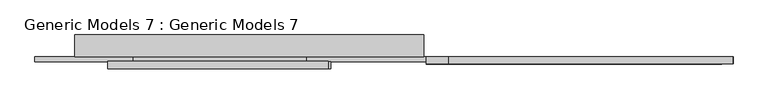
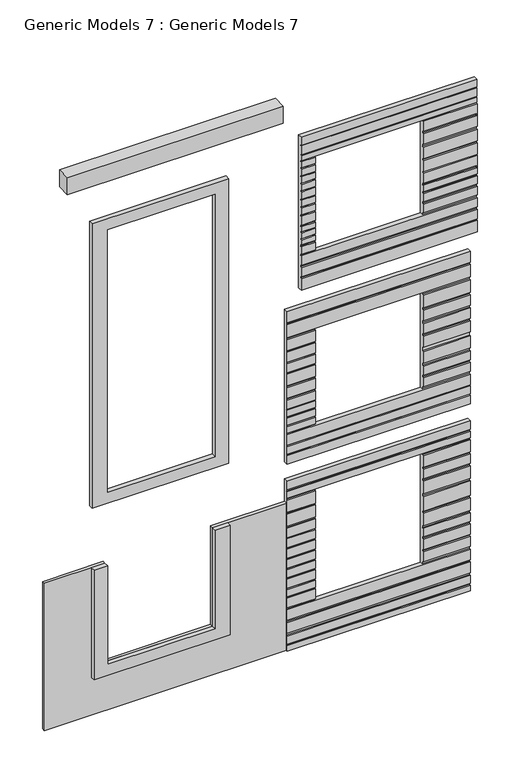
"""IFC4 building model written with IfcOpenShell, lengths in millimetres: proxy geometry, Generic Models 7 : Generic Models 7."""

from ifc_helpers import new_model, si_unit, frame, origin, place, context, project, spatial, polyline, outline, extrude, faceted_brep, source, transform, mapped, element, save


def generic_models_7_generic_models_7_680a3b92(model_context):
    return source(origin(), model_context, "Body", "SolidModel", [
        extrude(outline(polyline([(-16196.191855, -13854.1538163), (-19866.491855, -13854.1538163), (-19866.491855, -13625.5538163), (-16196.191855, -13625.5538163), (-16196.191855, -13854.1538163)])), frame((0.0, 0.0, 9448.8), z_axis=(0.0, 0.0, 1.0), x_axis=(1.0, 0.0, 0.0)), (0.0, 0.0, 1.0), 304.8),
        extrude(outline(polyline([(2645.3232141, -19485.491855), (675.8427781, -19485.491855), (675.8427781, -17174.091855), (2645.3232141, -17174.091855), (2645.3232141, -17428.091855), (874.5903603, -17428.091855), (874.5903603, -19256.891855), (2645.3232141, -19256.891855), (2645.3232141, -19485.491855)])), frame((0.0, -13981.1538163, 0.0), z_axis=(0.0, 1.0, 0.0), x_axis=(0.0, 0.0, 1.0)), (0.0, 0.0, 1.0), 76.2),
        faceted_brep([(-13059.291855, -13930.3538163, 3047.830136), (-16170.791855, -13930.3538163, 3047.830136), (-16170.791855, -13930.3538163, 2895.4466758), (-13059.291855, -13930.3538163, 2895.4466758), (-16170.791855, -13930.3538163, 0.0), (-13059.291855, -13930.3538163, 0.0), (-13059.291855, -13930.3538163, 95.1342014), (-16170.791855, -13930.3538163, 95.1342014), (-13859.391855, -13930.3538163, 2703.7494971), (-13859.391855, -13930.3538163, 2491.4485326), (-13059.291855, -13930.3538163, 2491.4485326), (-13059.291855, -13930.3538163, 2703.7494971), (-13859.391855, -13930.3538163, 2458.2818029), (-13859.391855, -13930.3538163, 2283.5976577), (-13059.291855, -13930.3538163, 2283.5976577), (-13059.291855, -13930.3538163, 2458.2818029), (-13859.391855, -13930.3538163, 2241.6081652), (-13859.391855, -13930.3538163, 2015.4004334), (-13059.291855, -13930.3538163, 2015.4004334), (-13059.291855, -13930.3538163, 2241.6081652), (-13859.391855, -13930.3538163, 1968.3766728), (-13859.391855, -13930.3538163, 1706.6714658), (-13059.291855, -13930.3538163, 1706.6714658), (-13059.291855, -13930.3538163, 1968.3766728), (-13859.391855, -13930.3538163, 1667.5135795), (-13859.391855, -13930.3538163, 1443.0083646), (-13059.291855, -13930.3538163, 1443.0083646), (-13059.291855, -13930.3538163, 1667.5135795), (-13859.391855, -13930.3538163, 1396.018901), (-13859.391855, -13930.3538163, 1241.8672624), (-13059.291855, -13930.3538163, 1241.8672624), (-13059.291855, -13930.3538163, 1396.018901), (-13859.391855, -13930.3538163, 978.3347801), (-13859.391855, -13930.3538163, 792.9874515), (-13059.291855, -13930.3538163, 792.9874515), (-13059.291855, -13930.3538163, 978.3347801), (-13859.391855, -13930.3538163, 1200.2294693), (-13859.391855, -13930.3538163, 1009.6610892), (-13059.291855, -13930.3538163, 1009.6610892), (-13059.291855, -13930.3538163, 1200.2294693), (-15688.191855, -13930.3538163, 2491.4485326), (-15688.191855, -13930.3538163, 2714.9644319), (-16170.791855, -13930.3538163, 2714.9644319), (-16170.791855, -13930.3538163, 2491.4485326), (-15688.191855, -13930.3538163, 2241.6081652), (-15688.191855, -13930.3538163, 2458.2818029), (-16170.791855, -13930.3538163, 2458.2818029), (-16170.791855, -13930.3538163, 2241.6081652), (-15688.191855, -13930.3538163, 2040.597682), (-15688.191855, -13930.3538163, 2205.0608046), (-16170.791855, -13930.3538163, 2205.0608046), (-16170.791855, -13930.3538163, 2040.597682), (-15688.191855, -13930.3538163, 1854.7223265), (-15688.191855, -13930.3538163, 2015.4004334), (-16170.791855, -13930.3538163, 2015.4004334), (-16170.791855, -13930.3538163, 1854.7223265), (-15688.191855, -13930.3538163, 1670.8505124), (-15688.191855, -13930.3538163, 1829.7520801), (-16170.791855, -13930.3538163, 1829.7520801), (-16170.791855, -13930.3538163, 1670.8505124), (-15688.191855, -13930.3538163, 1491.5187431), (-15688.191855, -13930.3538163, 1641.3402213), (-16170.791855, -13930.3538163, 1641.3402213), (-16170.791855, -13930.3538163, 1491.5187431), (-15688.191855, -13930.3538163, 1322.6616071), (-15688.191855, -13930.3538163, 1464.2784744), (-16170.791855, -13930.3538163, 1464.2784744), (-16170.791855, -13930.3538163, 1322.6616071), (-15688.191855, -13930.3538163, 1130.5851822), (-15688.191855, -13930.3538163, 1291.7567723), (-16170.791855, -13930.3538163, 1291.7567723), (-16170.791855, -13930.3538163, 1130.5851822), (-15688.191855, -13930.3538163, 776.4616885), (-15688.191855, -13930.3538163, 951.253413), (-16170.791855, -13930.3538163, 951.253413), (-16170.791855, -13930.3538163, 776.4616885), (-15688.191855, -13930.3538163, 978.4936817), (-15688.191855, -13930.3538163, 1105.6149359), (-16170.791855, -13930.3538163, 1105.6149359), (-16170.791855, -13930.3538163, 978.4936817), (-16170.791855, -13930.3538163, 512.7768801), (-16170.791855, -13930.3538163, 322.2032789), (-13059.291855, -13930.3538163, 322.2032789), (-13059.291855, -13930.3538163, 512.7768801), (-16170.791855, -13930.3538163, 270.5895953), (-16170.791855, -13930.3538163, 127.6593944), (-13059.291855, -13930.3538163, 127.6593944), (-13059.291855, -13930.3538163, 270.5895953), (-16170.791855, -13930.3538163, 2743.3706019), (-13059.291855, -13930.3538163, 2743.3706019), (-13059.291855, -13930.3538163, 2861.3685959), (-16170.791855, -13930.3538163, 2861.3685959), (-13059.291855, -13930.3538163, 741.3661492), (-16170.791855, -13930.3538163, 741.3661492), (-16170.791855, -13930.3538163, 556.4499971), (-13059.291855, -13930.3538163, 556.4499971), (-16170.791855, -13854.1538163, 3047.830136), (-13059.291855, -13854.1538163, 3047.830136), (-13059.291855, -13854.1538163, 0.0), (-16170.791855, -13854.1538163, 0.0), (-15688.191855, -13854.1538163, 2743.3706019), (-15688.191855, -13854.1538163, 741.3661492), (-13859.391855, -13854.1538163, 741.3661492), (-13859.391855, -13854.1538163, 2743.3706019), (-16170.791855, -13904.9538163, 95.1342014), (-16170.791855, -13904.9538163, 127.6593944), (-16170.791855, -13904.9538163, 270.5895953), (-16170.791855, -13904.9538163, 322.2032789), (-16170.791855, -13904.9538163, 512.7768801), (-16170.791855, -13904.9538163, 556.4499971), (-16170.791855, -13904.9538163, 741.3661492), (-16170.791855, -13904.9538163, 776.4616885), (-16170.791855, -13904.9538163, 951.253413), (-16170.791855, -13904.9538163, 978.4936817), (-16170.791855, -13904.9538163, 1105.6149359), (-16170.791855, -13904.9538163, 1130.5851822), (-16170.791855, -13904.9538163, 1291.7567723), (-16170.791855, -13904.9538163, 1322.6616071), (-16170.791855, -13904.9538163, 1464.2784744), (-16170.791855, -13904.9538163, 1491.5187431), (-16170.791855, -13904.9538163, 1641.3402213), (-16170.791855, -13904.9538163, 1670.8505124), (-16170.791855, -13904.9538163, 1829.7520801), (-16170.791855, -13904.9538163, 1854.7223265), (-16170.791855, -13904.9538163, 2015.4004334), (-16170.791855, -13904.9538163, 2040.597682), (-16170.791855, -13904.9538163, 2205.0608046), (-16170.791855, -13904.9538163, 2241.6081652), (-16170.791855, -13904.9538163, 2458.2818029), (-16170.791855, -13904.9538163, 2491.4485326), (-16170.791855, -13904.9538163, 2714.9644319), (-16170.791855, -13904.9538163, 2743.3706019), (-16170.791855, -13904.9538163, 2861.3685959), (-16170.791855, -13904.9538163, 2895.4466758), (-15688.191855, -13904.9538163, 2743.3706019), (-15688.191855, -13904.9538163, 2714.9644319), (-15688.191855, -13904.9538163, 2491.4485326), (-15688.191855, -13904.9538163, 2458.2818029), (-15688.191855, -13904.9538163, 2241.6081652), (-15688.191855, -13904.9538163, 2205.0608046), (-15688.191855, -13904.9538163, 2040.597682), (-15688.191855, -13904.9538163, 2015.4004334), (-15688.191855, -13904.9538163, 1854.7223265), (-15688.191855, -13904.9538163, 1829.7520801), (-15688.191855, -13904.9538163, 1670.8505124), (-15688.191855, -13904.9538163, 1641.3402213), (-15688.191855, -13904.9538163, 1491.5187431), (-15688.191855, -13904.9538163, 1464.2784744), (-15688.191855, -13904.9538163, 1322.6616071), (-15688.191855, -13904.9538163, 1291.7567723), (-15688.191855, -13904.9538163, 1130.5851822), (-15688.191855, -13904.9538163, 1105.6149359), (-15688.191855, -13904.9538163, 978.4936817), (-15688.191855, -13904.9538163, 951.253413), (-15688.191855, -13904.9538163, 776.4616885), (-15688.191855, -13904.9538163, 741.3661492), (-13859.391855, -13904.9538163, 2743.3706019), (-13059.291855, -13904.9538163, 2743.3706019), (-13059.291855, -13904.9538163, 2895.4466758), (-13059.291855, -13904.9538163, 2861.3685959), (-13059.291855, -13904.9538163, 2703.7494971), (-13059.291855, -13904.9538163, 2491.4485326), (-13059.291855, -13904.9538163, 2458.2818029), (-13059.291855, -13904.9538163, 2283.5976577), (-13059.291855, -13904.9538163, 2241.6081652), (-13059.291855, -13904.9538163, 2015.4004334), (-13059.291855, -13904.9538163, 1968.3766728), (-13059.291855, -13904.9538163, 1706.6714658), (-13059.291855, -13904.9538163, 1667.5135795), (-13059.291855, -13904.9538163, 1443.0083646), (-13059.291855, -13904.9538163, 1396.018901), (-13059.291855, -13904.9538163, 1241.8672624), (-13059.291855, -13904.9538163, 1200.2294693), (-13059.291855, -13904.9538163, 1009.6610892), (-13059.291855, -13904.9538163, 978.3347801), (-13059.291855, -13904.9538163, 792.9874515), (-13059.291855, -13904.9538163, 741.3661492), (-13059.291855, -13904.9538163, 556.4499971), (-13059.291855, -13904.9538163, 512.7768801), (-13059.291855, -13904.9538163, 322.2032789), (-13059.291855, -13904.9538163, 270.5895953), (-13059.291855, -13904.9538163, 127.6593944), (-13059.291855, -13904.9538163, 95.1342014), (-13859.391855, -13904.9538163, 741.3661492), (-13859.391855, -13904.9538163, 792.9874515), (-13859.391855, -13904.9538163, 978.3347801), (-13859.391855, -13904.9538163, 1009.6610892), (-13859.391855, -13904.9538163, 1200.2294693), (-13859.391855, -13904.9538163, 1241.8672624), (-13859.391855, -13904.9538163, 1396.018901), (-13859.391855, -13904.9538163, 1443.0083646), (-13859.391855, -13904.9538163, 1667.5135795), (-13859.391855, -13904.9538163, 1706.6714658), (-13859.391855, -13904.9538163, 1968.3766728), (-13859.391855, -13904.9538163, 2015.4004334), (-13859.391855, -13904.9538163, 2241.6081652), (-13859.391855, -13904.9538163, 2283.5976577), (-13859.391855, -13904.9538163, 2458.2818029), (-13859.391855, -13904.9538163, 2491.4485326), (-13859.391855, -13904.9538163, 2703.7494971)], [[[0, 1, 2, 3]], [[4, 5, 6, 7]], [[8, 9, 10, 11]], [[12, 13, 14, 15]], [[16, 17, 18, 19]], [[20, 21, 22, 23]], [[24, 25, 26, 27]], [[28, 29, 30, 31]], [[32, 33, 34, 35]], [[36, 37, 38, 39]], [[40, 41, 42, 43]], [[44, 45, 46, 47]], [[48, 49, 50, 51]], [[52, 53, 54, 55]], [[56, 57, 58, 59]], [[60, 61, 62, 63]], [[64, 65, 66, 67]], [[68, 69, 70, 71]], [[72, 73, 74, 75]], [[76, 77, 78, 79]], [[80, 81, 82, 83]], [[84, 85, 86, 87]], [[88, 89, 90, 91]], [[92, 93, 94, 95]], [[96, 97, 98, 99], [100, 101, 102, 103]], [[99, 4, 7, 104, 105, 85, 84, 106, 107, 81, 80, 108, 109, 94, 93, 110, 111, 75, 74, 112, 113, 79, 78, 114, 115, 71, 70, 116, 117, 67, 66, 118, 119, 63, 62, 120, 121, 59, 58, 122, 123, 55, 54, 124, 125, 51, 50, 126, 127, 47, 46, 128, 129, 43, 42, 130, 131, 88, 91, 132, 133, 2, 1, 96]], [[4, 99, 98, 5]], [[101, 100, 134, 135, 41, 40, 136, 137, 45, 44, 138, 139, 49, 48, 140, 141, 53, 52, 142, 143, 57, 56, 144, 145, 61, 60, 146, 147, 65, 64, 148, 149, 69, 68, 150, 151, 77, 76, 152, 153, 73, 72, 154, 155]], [[1, 0, 97, 96]], [[88, 131, 134, 100, 103, 156, 157, 89]], [[97, 0, 3, 158, 159, 90, 89, 157, 160, 11, 10, 161, 162, 15, 14, 163, 164, 19, 18, 165, 166, 23, 22, 167, 168, 27, 26, 169, 170, 31, 30, 171, 172, 39, 38, 173, 174, 35, 34, 175, 176, 92, 95, 177, 178, 83, 82, 179, 180, 87, 86, 181, 182, 6, 5, 98]], [[92, 176, 183, 102, 101, 155, 110, 93]], [[103, 102, 183, 184, 33, 32, 185, 186, 37, 36, 187, 188, 29, 28, 189, 190, 25, 24, 191, 192, 21, 20, 193, 194, 17, 16, 195, 196, 13, 12, 197, 198, 9, 8, 199, 156]], [[157, 156, 199, 160]], [[110, 155, 154, 111]], [[158, 133, 132, 159]], [[130, 135, 134, 131]], [[136, 129, 128, 137]], [[138, 127, 126, 139]], [[140, 125, 124, 141]], [[142, 123, 122, 143]], [[144, 121, 120, 145]], [[146, 119, 118, 147]], [[148, 117, 116, 149]], [[150, 115, 114, 151]], [[152, 113, 112, 153]], [[161, 198, 197, 162]], [[163, 196, 195, 164]], [[165, 194, 193, 166]], [[167, 192, 191, 168]], [[175, 184, 183, 176]], [[169, 190, 189, 170]], [[171, 188, 187, 172]], [[173, 186, 185, 174]], [[177, 109, 108, 178]], [[179, 107, 106, 180]], [[181, 105, 104, 182]], [[159, 132, 91, 90]], [[133, 158, 3, 2]], [[135, 130, 42, 41]], [[160, 199, 8, 11]], [[137, 128, 46, 45]], [[129, 136, 40, 43]], [[139, 126, 50, 49]], [[127, 138, 44, 47]], [[141, 124, 54, 53]], [[125, 140, 48, 51]], [[143, 122, 58, 57]], [[123, 142, 52, 55]], [[145, 120, 62, 61]], [[121, 144, 56, 59]], [[147, 118, 66, 65]], [[119, 146, 60, 63]], [[111, 154, 72, 75]], [[149, 116, 70, 69]], [[117, 148, 64, 67]], [[151, 114, 78, 77]], [[115, 150, 68, 71]], [[153, 112, 74, 73]], [[113, 152, 76, 79]], [[162, 197, 12, 15]], [[198, 161, 10, 9]], [[164, 195, 16, 19]], [[196, 163, 14, 13]], [[166, 193, 20, 23]], [[194, 165, 18, 17]], [[168, 191, 24, 27]], [[192, 167, 22, 21]], [[184, 175, 34, 33]], [[170, 189, 28, 31]], [[190, 169, 26, 25]], [[172, 187, 36, 39]], [[188, 171, 30, 29]], [[174, 185, 32, 35]], [[186, 173, 38, 37]], [[178, 108, 80, 83]], [[109, 177, 95, 94]], [[180, 106, 84, 87]], [[107, 179, 82, 81]], [[182, 104, 7, 6]], [[105, 181, 86, 85]]]),
        faceted_brep([(-13059.291855, -13930.3538163, 6096.0), (-16170.791855, -13930.3538163, 6096.0), (-16170.791855, -13930.3538163, 5900.4772221), (-13059.291855, -13930.3538163, 5900.4772221), (-16170.791855, -13930.3538163, 3352.8), (-13059.291855, -13930.3538163, 3352.8), (-13059.291855, -13930.3538163, 3510.1812657), (-16170.791855, -13930.3538163, 3510.1812657), (-13859.391855, -13930.3538163, 5586.1430956), (-13859.391855, -13930.3538163, 5358.1855285), (-13059.291855, -13930.3538163, 5358.1855285), (-13059.291855, -13930.3538163, 5586.1430956), (-13859.391855, -13930.3538163, 5316.1560639), (-13859.391855, -13930.3538163, 5121.0192637), (-13059.291855, -13930.3538163, 5121.0192637), (-13059.291855, -13930.3538163, 5316.1560639), (-13859.391855, -13930.3538163, 5075.9876944), (-13859.391855, -13930.3538163, 4892.8593127), (-13059.291855, -13930.3538163, 4892.8593127), (-13059.291855, -13930.3538163, 5075.9876944), (-13859.391855, -13930.3538163, 4847.8277434), (-13859.391855, -13930.3538163, 4647.2829369), (-13059.291855, -13930.3538163, 4647.2829369), (-13059.291855, -13930.3538163, 4847.8277434), (-13859.391855, -13930.3538163, 4572.0), (-13859.391855, -13930.3538163, 4358.4846906), (-13059.291855, -13930.3538163, 4358.4846906), (-13059.291855, -13930.3538163, 4572.0), (-13859.391855, -13930.3538163, 4103.305798), (-13859.391855, -13930.3538163, 3938.190044), (-13059.291855, -13930.3538163, 3938.190044), (-13059.291855, -13930.3538163, 4103.305798), (-13859.391855, -13930.3538163, 4307.4489121), (-13859.391855, -13930.3538163, 4145.3352627), (-13059.291855, -13930.3538163, 4145.3352627), (-13059.291855, -13930.3538163, 4307.4489121), (-15688.191855, -13930.3538163, 5394.7918514), (-15688.191855, -13930.3538163, 5596.5851986), (-16170.791855, -13930.3538163, 5596.5851986), (-16170.791855, -13930.3538163, 5394.7918514), (-15688.191855, -13930.3538163, 5189.2435919), (-15688.191855, -13930.3538163, 5368.6865939), (-16170.791855, -13930.3538163, 5368.6865939), (-16170.791855, -13930.3538163, 5189.2435919), (-15688.191855, -13930.3538163, 5003.2129882), (-15688.191855, -13930.3538163, 5165.065585), (-16170.791855, -13930.3538163, 5165.065585), (-16170.791855, -13930.3538163, 5003.2129882), (-15688.191855, -13930.3538163, 4768.0829809), (-15688.191855, -13930.3538163, 4971.8866791), (-16170.791855, -13930.3538163, 4971.8866791), (-16170.791855, -13930.3538163, 4768.0829809), (-15688.191855, -13930.3538163, 4543.4835442), (-15688.191855, -13930.3538163, 4734.1666909), (-16170.791855, -13930.3538163, 4734.1666909), (-16170.791855, -13930.3538163, 4543.4835442), (-15688.191855, -13930.3538163, 4346.2982993), (-15688.191855, -13930.3538163, 4510.8707461), (-16170.791855, -13930.3538163, 4510.8707461), (-16170.791855, -13930.3538163, 4346.2982993), (-15688.191855, -13930.3538163, 4212.2061738), (-15688.191855, -13930.3538163, 4324.3827349), (-16170.791855, -13930.3538163, 4324.3827349), (-16170.791855, -13930.3538163, 4212.2061738), (-15688.191855, -13930.3538163, 3915.2580645), (-15688.191855, -13930.3538163, 4034.0671597), (-16170.791855, -13930.3538163, 4034.0671597), (-16170.791855, -13930.3538163, 3915.2580645), (-15688.191855, -13930.3538163, 4059.1404662), (-15688.191855, -13930.3538163, 4183.0263018), (-16170.791855, -13930.3538163, 4183.0263018), (-16170.791855, -13930.3538163, 4059.1404662), (-16170.791855, -13930.3538163, 3674.3162613), (-16170.791855, -13930.3538163, 3536.2157608), (-13059.291855, -13930.3538163, 3536.2157608), (-13059.291855, -13930.3538163, 3674.3162613), (-16170.791855, -13930.3538163, 5631.310527), (-13059.291855, -13930.3538163, 5631.310527), (-13059.291855, -13930.3538163, 5862.3466577), (-16170.791855, -13930.3538163, 5862.3466577), (-13059.291855, -13930.3538163, 3888.7401376), (-16170.791855, -13930.3538163, 3888.7401376), (-16170.791855, -13930.3538163, 3697.1052355), (-13059.291855, -13930.3538163, 3697.1052355), (-16170.791855, -13854.1538163, 6096.0), (-13059.291855, -13854.1538163, 6096.0), (-13059.291855, -13854.1538163, 3352.8), (-16170.791855, -13854.1538163, 3352.8), (-15688.191855, -13854.1538163, 5631.310527), (-15688.191855, -13854.1538163, 3888.7401376), (-13859.391855, -13854.1538163, 3888.7401376), (-13859.391855, -13854.1538163, 5631.310527), (-16170.791855, -13904.9538163, 3510.1812657), (-16170.791855, -13904.9538163, 3536.2157608), (-16170.791855, -13904.9538163, 3674.3162613), (-16170.791855, -13904.9538163, 3697.1052355), (-16170.791855, -13904.9538163, 3888.7401376), (-16170.791855, -13904.9538163, 3915.2580645), (-16170.791855, -13904.9538163, 4034.0671597), (-16170.791855, -13904.9538163, 4059.1404662), (-16170.791855, -13904.9538163, 4183.0263018), (-16170.791855, -13904.9538163, 4212.2061738), (-16170.791855, -13904.9538163, 4324.3827349), (-16170.791855, -13904.9538163, 4346.2982993), (-16170.791855, -13904.9538163, 4510.8707461), (-16170.791855, -13904.9538163, 4543.4835442), (-16170.791855, -13904.9538163, 4734.1666909), (-16170.791855, -13904.9538163, 4768.0829809), (-16170.791855, -13904.9538163, 4971.8866791), (-16170.791855, -13904.9538163, 5003.2129882), (-16170.791855, -13904.9538163, 5165.065585), (-16170.791855, -13904.9538163, 5189.2435919), (-16170.791855, -13904.9538163, 5368.6865939), (-16170.791855, -13904.9538163, 5394.7918514), (-16170.791855, -13904.9538163, 5596.5851986), (-16170.791855, -13904.9538163, 5631.310527), (-16170.791855, -13904.9538163, 5862.3466577), (-16170.791855, -13904.9538163, 5900.4772221), (-15688.191855, -13904.9538163, 5631.310527), (-15688.191855, -13904.9538163, 5596.5851986), (-15688.191855, -13904.9538163, 5394.7918514), (-15688.191855, -13904.9538163, 5368.6865939), (-15688.191855, -13904.9538163, 5189.2435919), (-15688.191855, -13904.9538163, 5165.065585), (-15688.191855, -13904.9538163, 5003.2129882), (-15688.191855, -13904.9538163, 4971.8866791), (-15688.191855, -13904.9538163, 4768.0829809), (-15688.191855, -13904.9538163, 4734.1666909), (-15688.191855, -13904.9538163, 4543.4835442), (-15688.191855, -13904.9538163, 4510.8707461), (-15688.191855, -13904.9538163, 4346.2982993), (-15688.191855, -13904.9538163, 4324.3827349), (-15688.191855, -13904.9538163, 4212.2061738), (-15688.191855, -13904.9538163, 4183.0263018), (-15688.191855, -13904.9538163, 4059.1404662), (-15688.191855, -13904.9538163, 4034.0671597), (-15688.191855, -13904.9538163, 3915.2580645), (-15688.191855, -13904.9538163, 3888.7401376), (-13859.391855, -13904.9538163, 5631.310527), (-13059.291855, -13904.9538163, 5631.310527), (-13059.291855, -13904.9538163, 5900.4772221), (-13059.291855, -13904.9538163, 5862.3466577), (-13059.291855, -13904.9538163, 5586.1430956), (-13059.291855, -13904.9538163, 5358.1855285), (-13059.291855, -13904.9538163, 5316.1560639), (-13059.291855, -13904.9538163, 5121.0192637), (-13059.291855, -13904.9538163, 5075.9876944), (-13059.291855, -13904.9538163, 4892.8593127), (-13059.291855, -13904.9538163, 4847.8277434), (-13059.291855, -13904.9538163, 4647.2829369), (-13059.291855, -13904.9538163, 4572.0), (-13059.291855, -13904.9538163, 4358.4846906), (-13059.291855, -13904.9538163, 4307.4489121), (-13059.291855, -13904.9538163, 4145.3352627), (-13059.291855, -13904.9538163, 4103.305798), (-13059.291855, -13904.9538163, 3938.190044), (-13059.291855, -13904.9538163, 3888.7401376), (-13059.291855, -13904.9538163, 3697.1052355), (-13059.291855, -13904.9538163, 3674.3162613), (-13059.291855, -13904.9538163, 3536.2157608), (-13059.291855, -13904.9538163, 3510.1812657), (-13859.391855, -13904.9538163, 3888.7401376), (-13859.391855, -13904.9538163, 3938.190044), (-13859.391855, -13904.9538163, 4103.305798), (-13859.391855, -13904.9538163, 4145.3352627), (-13859.391855, -13904.9538163, 4307.4489121), (-13859.391855, -13904.9538163, 4358.4846906), (-13859.391855, -13904.9538163, 4572.0), (-13859.391855, -13904.9538163, 4647.2829369), (-13859.391855, -13904.9538163, 4847.8277434), (-13859.391855, -13904.9538163, 4892.8593127), (-13859.391855, -13904.9538163, 5075.9876944), (-13859.391855, -13904.9538163, 5121.0192637), (-13859.391855, -13904.9538163, 5316.1560639), (-13859.391855, -13904.9538163, 5358.1855285), (-13859.391855, -13904.9538163, 5586.1430956)], [[[0, 1, 2, 3]], [[4, 5, 6, 7]], [[8, 9, 10, 11]], [[12, 13, 14, 15]], [[16, 17, 18, 19]], [[20, 21, 22, 23]], [[24, 25, 26, 27]], [[28, 29, 30, 31]], [[32, 33, 34, 35]], [[36, 37, 38, 39]], [[40, 41, 42, 43]], [[44, 45, 46, 47]], [[48, 49, 50, 51]], [[52, 53, 54, 55]], [[56, 57, 58, 59]], [[60, 61, 62, 63]], [[64, 65, 66, 67]], [[68, 69, 70, 71]], [[72, 73, 74, 75]], [[76, 77, 78, 79]], [[80, 81, 82, 83]], [[84, 85, 86, 87], [88, 89, 90, 91]], [[87, 4, 7, 92, 93, 73, 72, 94, 95, 82, 81, 96, 97, 67, 66, 98, 99, 71, 70, 100, 101, 63, 62, 102, 103, 59, 58, 104, 105, 55, 54, 106, 107, 51, 50, 108, 109, 47, 46, 110, 111, 43, 42, 112, 113, 39, 38, 114, 115, 76, 79, 116, 117, 2, 1, 84]], [[4, 87, 86, 5]], [[89, 88, 118, 119, 37, 36, 120, 121, 41, 40, 122, 123, 45, 44, 124, 125, 49, 48, 126, 127, 53, 52, 128, 129, 57, 56, 130, 131, 61, 60, 132, 133, 69, 68, 134, 135, 65, 64, 136, 137]], [[1, 0, 85, 84]], [[76, 115, 118, 88, 91, 138, 139, 77]], [[85, 0, 3, 140, 141, 78, 77, 139, 142, 11, 10, 143, 144, 15, 14, 145, 146, 19, 18, 147, 148, 23, 22, 149, 150, 27, 26, 151, 152, 35, 34, 153, 154, 31, 30, 155, 156, 80, 83, 157, 158, 75, 74, 159, 160, 6, 5, 86]], [[80, 156, 161, 90, 89, 137, 96, 81]], [[91, 90, 161, 162, 29, 28, 163, 164, 33, 32, 165, 166, 25, 24, 167, 168, 21, 20, 169, 170, 17, 16, 171, 172, 13, 12, 173, 174, 9, 8, 175, 138]], [[139, 138, 175, 142]], [[96, 137, 136, 97]], [[140, 117, 116, 141]], [[114, 119, 118, 115]], [[120, 113, 112, 121]], [[122, 111, 110, 123]], [[124, 109, 108, 125]], [[126, 107, 106, 127]], [[128, 105, 104, 129]], [[130, 103, 102, 131]], [[132, 101, 100, 133]], [[134, 99, 98, 135]], [[143, 174, 173, 144]], [[145, 172, 171, 146]], [[147, 170, 169, 148]], [[149, 168, 167, 150]], [[151, 166, 165, 152]], [[155, 162, 161, 156]], [[153, 164, 163, 154]], [[157, 95, 94, 158]], [[159, 93, 92, 160]], [[141, 116, 79, 78]], [[117, 140, 3, 2]], [[119, 114, 38, 37]], [[142, 175, 8, 11]], [[121, 112, 42, 41]], [[113, 120, 36, 39]], [[123, 110, 46, 45]], [[111, 122, 40, 43]], [[125, 108, 50, 49]], [[109, 124, 44, 47]], [[127, 106, 54, 53]], [[107, 126, 48, 51]], [[129, 104, 58, 57]], [[105, 128, 52, 55]], [[131, 102, 62, 61]], [[103, 130, 56, 59]], [[97, 136, 64, 67]], [[133, 100, 70, 69]], [[101, 132, 60, 63]], [[135, 98, 66, 65]], [[99, 134, 68, 71]], [[144, 173, 12, 15]], [[174, 143, 10, 9]], [[146, 171, 16, 19]], [[172, 145, 14, 13]], [[148, 169, 20, 23]], [[170, 147, 18, 17]], [[150, 167, 24, 27]], [[168, 149, 22, 21]], [[152, 165, 32, 35]], [[166, 151, 26, 25]], [[162, 155, 30, 29]], [[154, 163, 28, 31]], [[164, 153, 34, 33]], [[158, 94, 72, 75]], [[95, 157, 83, 82]], [[160, 92, 7, 6]], [[93, 159, 74, 73]]]),
        faceted_brep([(-12944.991855, -13930.3538163, 9144.0), (-15932.2432214, -13930.3538163, 9144.0), (-15932.2432214, -13930.3538163, 9006.4899372), (-12944.991855, -13930.3538163, 9006.4899372), (-15932.2432214, -13930.3538163, 6400.8), (-12942.3480642, -13930.3538163, 6400.8), (-12942.3480642, -13930.3538163, 6605.0090514), (-15932.2432214, -13930.3538163, 6605.0090514), (-13859.391855, -13930.3538163, 8705.0077655), (-13859.391855, -13930.3538163, 8531.3898217), (-12944.991855, -13930.3538163, 8531.3898217), (-12944.991855, -13930.3538163, 8486.3582524), (-13859.391855, -13930.3538163, 8486.3582524), (-13859.391855, -13930.3538163, 8297.9712056), (-12942.3480642, -13930.3538163, 8297.9712056), (-12942.3480642, -13930.3538163, 8705.0077655), (-13859.391855, -13930.3538163, 8246.1898829), (-13859.391855, -13930.3538163, 8036.0425596), (-12942.3480642, -13930.3538163, 8036.0425596), (-12942.3480642, -13930.3538163, 8246.1898829), (-13859.391855, -13930.3538163, 8003.0194088), (-13859.391855, -13930.3538163, 7798.8762948), (-12942.3480642, -13930.3538163, 7798.8762948), (-12942.3480642, -13930.3538163, 8003.0194088), (-13859.391855, -13930.3538163, 7777.8615625), (-13859.391855, -13930.3538163, 7594.7331807), (-12944.991855, -13930.3538163, 7594.7331807), (-12944.991855, -13930.3538163, 7556.5), (-13859.391855, -13930.3538163, 7556.5), (-13859.391855, -13930.3538163, 7443.1279816), (-12942.3480642, -13930.3538163, 7443.1279816), (-12942.3480642, -13930.3538163, 7777.8615625), (-13859.391855, -13930.3538163, 7219.2359457), (-13859.391855, -13930.3538163, 7069.3648725), (-12942.3480642, -13930.3538163, 7069.3648725), (-12942.3480642, -13930.3538163, 7219.2359457), (-13859.391855, -13930.3538163, 7405.6005898), (-13859.391855, -13930.3538163, 7264.5016727), (-12942.3480642, -13930.3538163, 7264.5016727), (-12942.3480642, -13930.3538163, 7405.6005898), (-15688.191855, -13930.3538163, 8595.4203116), (-15688.191855, -13930.3538163, 8703.5574843), (-15932.2432214, -13930.3538163, 8703.5574843), (-15932.2432214, -13930.3538163, 8595.4203116), (-15688.191855, -13930.3538163, 8454.6703408), (-15688.191855, -13930.3538163, 8571.3898288), (-15932.2432214, -13930.3538163, 8571.3898288), (-15932.2432214, -13930.3538163, 8454.6703408), (-15688.191855, -13930.3538163, 8320.7862221), (-15688.191855, -13930.3538163, 8434.0727841), (-15932.2432214, -13930.3538163, 8434.0727841), (-15932.2432214, -13930.3538163, 8320.7862221), (-15688.191855, -13930.3538163, 8181.7527143), (-15688.191855, -13930.3538163, 8297.9712056), (-15932.2432214, -13930.3538163, 8297.9712056), (-15932.2432214, -13930.3538163, 8181.7527143), (-15688.191855, -13930.3538163, 8028.9875021), (-15688.191855, -13930.3538163, 8159.4386946), (-15932.2432214, -13930.3538163, 8159.4386946), (-15932.2432214, -13930.3538163, 8028.9875021), (-15688.191855, -13930.3538163, 7896.8198465), (-15688.191855, -13930.3538163, 8013.5393345), (-15932.2432214, -13930.3538163, 8013.5393345), (-15932.2432214, -13930.3538163, 7896.8198465), (-15688.191855, -13930.3538163, 7752.6369495), (-15688.191855, -13930.3538163, 7870.5495936), (-15932.2432214, -13930.3538163, 7870.5495936), (-15932.2432214, -13930.3538163, 7752.6369495), (-15688.191855, -13930.3538163, 7570.6578745), (-15688.191855, -13930.3538163, 7725.553622), (-15932.2432214, -13930.3538163, 7725.553622), (-15932.2432214, -13930.3538163, 7570.6578745), (-15688.191855, -13930.3538163, 7041.7426563), (-15688.191855, -13930.3538163, 7177.944), (-15932.2432214, -13930.3538163, 7177.944), (-15932.2432214, -13930.3538163, 7041.7426563), (-15688.191855, -13930.3538163, 7215.576811), (-15688.191855, -13930.3538163, 7300.8337996), (-15932.2432214, -13930.3538163, 7300.8337996), (-15932.2432214, -13930.3538163, 7215.576811), (-15688.191855, -13930.3538163, 7447.1063038), (-15688.191855, -13930.3538163, 7536.6075385), (-15932.2432214, -13930.3538163, 7536.6075385), (-15932.2432214, -13930.3538163, 7447.1063038), (-15688.191855, -13930.3538163, 7324.7150248), (-15688.191855, -13930.3538163, 7423.2250786), (-15932.2432214, -13930.3538163, 7423.2250786), (-15932.2432214, -13930.3538163, 7324.7150248), (-15932.2432214, -13930.3538163, 8992.2048185), (-15932.2432214, -13930.3538163, 8836.7725259), (-12944.991855, -13930.3538163, 8836.7725259), (-12944.991855, -13930.3538163, 8992.2048185), (-15932.2432214, -13930.3538163, 6806.8826886), (-15932.2432214, -13930.3538163, 6637.7319917), (-12942.3480642, -13930.3538163, 6637.7319917), (-12942.3480642, -13930.3538163, 6806.8826886), (-15932.2432214, -13930.3538163, 8725.3928177), (-12944.991855, -13930.3538163, 8725.3928177), (-12944.991855, -13930.3538163, 8818.4435851), (-15932.2432214, -13930.3538163, 8818.4435851), (-12942.3480642, -13930.3538163, 7015.7063696), (-15932.2432214, -13930.3538163, 7015.7063696), (-15932.2432214, -13930.3538163, 6847.5664272), (-12942.3480642, -13930.3538163, 6847.5664272), (-12944.991855, -13854.1538163, 9144.0), (-12944.991855, -13854.1538163, 8725.3928177), (-12942.3480642, -13854.1538163, 8725.3928177), (-12942.3480642, -13854.1538163, 6400.8), (-15932.2432214, -13854.1538163, 6400.8), (-15932.2432214, -13854.1538163, 9144.0), (-15688.191855, -13854.1538163, 8725.3928177), (-15688.191855, -13854.1538163, 7015.7063696), (-13859.391855, -13854.1538163, 7015.7063696), (-13859.391855, -13854.1538163, 8725.3928177), (-15932.2432214, -13904.9538163, 6605.0090514), (-15932.2432214, -13904.9538163, 6637.7319917), (-15932.2432214, -13904.9538163, 6806.8826886), (-15932.2432214, -13904.9538163, 6847.5664272), (-15932.2432214, -13904.9538163, 7015.7063696), (-15932.2432214, -13904.9538163, 7041.7426563), (-15932.2432214, -13904.9538163, 7177.944), (-15932.2432214, -13904.9538163, 7215.576811), (-15932.2432214, -13904.9538163, 7300.8337996), (-15932.2432214, -13904.9538163, 7324.7150248), (-15932.2432214, -13904.9538163, 7423.2250786), (-15932.2432214, -13904.9538163, 7447.1063038), (-15932.2432214, -13904.9538163, 7536.6075385), (-15932.2432214, -13904.9538163, 7570.6578745), (-15932.2432214, -13904.9538163, 7725.553622), (-15932.2432214, -13904.9538163, 7752.6369495), (-15932.2432214, -13904.9538163, 7870.5495936), (-15932.2432214, -13904.9538163, 7896.8198465), (-15932.2432214, -13904.9538163, 8013.5393345), (-15932.2432214, -13904.9538163, 8028.9875021), (-15932.2432214, -13904.9538163, 8159.4386946), (-15932.2432214, -13904.9538163, 8181.7527143), (-15932.2432214, -13904.9538163, 8297.9712056), (-15932.2432214, -13904.9538163, 8320.7862221), (-15932.2432214, -13904.9538163, 8434.0727841), (-15932.2432214, -13904.9538163, 8454.6703408), (-15932.2432214, -13904.9538163, 8571.3898288), (-15932.2432214, -13904.9538163, 8595.4203116), (-15932.2432214, -13904.9538163, 8703.5574843), (-15932.2432214, -13904.9538163, 8725.3928177), (-15932.2432214, -13904.9538163, 8818.4435851), (-15932.2432214, -13904.9538163, 8836.7725259), (-15932.2432214, -13904.9538163, 8992.2048185), (-15932.2432214, -13904.9538163, 9006.4899372), (-15688.191855, -13904.9538163, 8725.3928177), (-15688.191855, -13904.9538163, 8703.5574843), (-15688.191855, -13904.9538163, 8595.4203116), (-15688.191855, -13904.9538163, 8571.3898288), (-15688.191855, -13904.9538163, 8454.6703408), (-15688.191855, -13904.9538163, 8434.0727841), (-15688.191855, -13904.9538163, 8320.7862221), (-15688.191855, -13904.9538163, 8297.9712056), (-15688.191855, -13904.9538163, 8181.7527143), (-15688.191855, -13904.9538163, 8159.4386946), (-15688.191855, -13904.9538163, 8028.9875021), (-15688.191855, -13904.9538163, 8013.5393345), (-15688.191855, -13904.9538163, 7896.8198465), (-15688.191855, -13904.9538163, 7870.5495936), (-15688.191855, -13904.9538163, 7752.6369495), (-15688.191855, -13904.9538163, 7725.553622), (-15688.191855, -13904.9538163, 7570.6578745), (-15688.191855, -13904.9538163, 7536.6075385), (-15688.191855, -13904.9538163, 7447.1063038), (-15688.191855, -13904.9538163, 7423.2250786), (-15688.191855, -13904.9538163, 7324.7150248), (-15688.191855, -13904.9538163, 7300.8337996), (-15688.191855, -13904.9538163, 7215.576811), (-15688.191855, -13904.9538163, 7177.944), (-15688.191855, -13904.9538163, 7041.7426563), (-15688.191855, -13904.9538163, 7015.7063696), (-13859.391855, -13904.9538163, 8725.3928177), (-12944.991855, -13904.9538163, 8725.3928177), (-12944.991855, -13904.9538163, 9006.4899372), (-12944.991855, -13904.9538163, 8992.2048185), (-12944.991855, -13904.9538163, 8836.7725259), (-12944.991855, -13904.9538163, 8818.4435851), (-12942.3480642, -13904.9538163, 7015.7063696), (-13859.391855, -13904.9538163, 7015.7063696), (-12942.3480642, -13904.9538163, 8725.3928177), (-12942.3480642, -13904.9538163, 8705.0077655), (-12942.3480642, -13904.9538163, 8297.9712056), (-12942.3480642, -13904.9538163, 8246.1898829), (-12942.3480642, -13904.9538163, 8036.0425596), (-12942.3480642, -13904.9538163, 8003.0194088), (-12942.3480642, -13904.9538163, 7798.8762948), (-12942.3480642, -13904.9538163, 7777.8615625), (-12942.3480642, -13904.9538163, 7443.1279816), (-12942.3480642, -13904.9538163, 7405.6005898), (-12942.3480642, -13904.9538163, 7264.5016727), (-12942.3480642, -13904.9538163, 7219.2359457), (-12942.3480642, -13904.9538163, 7069.3648725), (-12942.3480642, -13904.9538163, 6847.5664272), (-12942.3480642, -13904.9538163, 6806.8826886), (-12942.3480642, -13904.9538163, 6637.7319917), (-12942.3480642, -13904.9538163, 6605.0090514), (-13859.391855, -13904.9538163, 7069.3648725), (-13859.391855, -13904.9538163, 7219.2359457), (-13859.391855, -13904.9538163, 7264.5016727), (-13859.391855, -13904.9538163, 7405.6005898), (-13859.391855, -13904.9538163, 7443.1279816), (-13859.391855, -13904.9538163, 7556.5), (-13859.391855, -13904.9538163, 7594.7331807), (-13859.391855, -13904.9538163, 7777.8615625), (-13859.391855, -13904.9538163, 7798.8762948), (-13859.391855, -13904.9538163, 8003.0194088), (-13859.391855, -13904.9538163, 8036.0425596), (-13859.391855, -13904.9538163, 8246.1898829), (-13859.391855, -13904.9538163, 8297.9712056), (-13859.391855, -13904.9538163, 8486.3582524), (-13859.391855, -13904.9538163, 8531.3898217), (-13859.391855, -13904.9538163, 8705.0077655), (-12944.991855, -13904.9538163, 8531.3898217), (-12944.991855, -13904.9538163, 8486.3582524), (-12944.991855, -13904.9538163, 7594.7331807), (-12944.991855, -13904.9538163, 7556.5)], [[[0, 1, 2, 3]], [[4, 5, 6, 7]], [[8, 9, 10, 11, 12, 13, 14, 15]], [[16, 17, 18, 19]], [[20, 21, 22, 23]], [[24, 25, 26, 27, 28, 29, 30, 31]], [[32, 33, 34, 35]], [[36, 37, 38, 39]], [[40, 41, 42, 43]], [[44, 45, 46, 47]], [[48, 49, 50, 51]], [[52, 53, 54, 55]], [[56, 57, 58, 59]], [[60, 61, 62, 63]], [[64, 65, 66, 67]], [[68, 69, 70, 71]], [[72, 73, 74, 75]], [[76, 77, 78, 79]], [[80, 81, 82, 83]], [[84, 85, 86, 87]], [[88, 89, 90, 91]], [[92, 93, 94, 95]], [[96, 97, 98, 99]], [[100, 101, 102, 103]], [[104, 105, 106, 107, 108, 109], [110, 111, 112, 113]], [[108, 4, 7, 114, 115, 93, 92, 116, 117, 102, 101, 118, 119, 75, 74, 120, 121, 79, 78, 122, 123, 87, 86, 124, 125, 83, 82, 126, 127, 71, 70, 128, 129, 67, 66, 130, 131, 63, 62, 132, 133, 59, 58, 134, 135, 55, 54, 136, 137, 51, 50, 138, 139, 47, 46, 140, 141, 43, 42, 142, 143, 96, 99, 144, 145, 89, 88, 146, 147, 2, 1, 109]], [[4, 108, 107, 5]], [[111, 110, 148, 149, 41, 40, 150, 151, 45, 44, 152, 153, 49, 48, 154, 155, 53, 52, 156, 157, 57, 56, 158, 159, 61, 60, 160, 161, 65, 64, 162, 163, 69, 68, 164, 165, 81, 80, 166, 167, 85, 84, 168, 169, 77, 76, 170, 171, 73, 72, 172, 173]], [[1, 0, 104, 109]], [[96, 143, 148, 110, 113, 174, 175, 97]], [[105, 104, 0, 3, 176, 177, 91, 90, 178, 179, 98, 97, 175]], [[100, 180, 181, 112, 111, 173, 118, 101]], [[5, 107, 106, 182, 183, 15, 14, 184, 185, 19, 18, 186, 187, 23, 22, 188, 189, 31, 30, 190, 191, 39, 38, 192, 193, 35, 34, 194, 180, 100, 103, 195, 196, 95, 94, 197, 198, 6]], [[106, 105, 175, 182]], [[113, 112, 181, 199, 33, 32, 200, 201, 37, 36, 202, 203, 29, 28, 204, 205, 25, 24, 206, 207, 21, 20, 208, 209, 17, 16, 210, 211, 13, 12, 212, 213, 9, 8, 214, 174]], [[118, 173, 172, 119]], [[176, 147, 146, 177]], [[178, 145, 144, 179]], [[214, 183, 182, 175, 174]], [[150, 141, 140, 151]], [[152, 139, 138, 153]], [[154, 137, 136, 155]], [[156, 135, 134, 157]], [[158, 133, 132, 159]], [[160, 131, 130, 161]], [[162, 129, 128, 163]], [[164, 127, 126, 165]], [[120, 171, 170, 121]], [[124, 167, 166, 125]], [[215, 213, 212, 216]], [[184, 211, 210, 185]], [[186, 209, 208, 187]], [[188, 207, 206, 189]], [[217, 205, 204, 218]], [[194, 199, 181, 180]], [[190, 203, 202, 191]], [[192, 201, 200, 193]], [[195, 117, 116, 196]], [[197, 115, 114, 198]], [[142, 149, 148, 143]], [[122, 169, 168, 123]], [[177, 146, 88, 91]], [[147, 176, 3, 2]], [[179, 144, 99, 98]], [[145, 178, 90, 89]], [[183, 214, 8, 15]], [[149, 142, 42, 41]], [[151, 140, 46, 45]], [[141, 150, 40, 43]], [[153, 138, 50, 49]], [[139, 152, 44, 47]], [[155, 136, 54, 53]], [[137, 154, 48, 51]], [[157, 134, 58, 57]], [[135, 156, 52, 55]], [[159, 132, 62, 61]], [[133, 158, 56, 59]], [[161, 130, 66, 65]], [[131, 160, 60, 63]], [[163, 128, 70, 69]], [[129, 162, 64, 67]], [[165, 126, 82, 81]], [[127, 164, 68, 71]], [[119, 172, 72, 75]], [[121, 170, 76, 79]], [[171, 120, 74, 73]], [[123, 168, 84, 87]], [[169, 122, 78, 77]], [[125, 166, 80, 83]], [[167, 124, 86, 85]], [[215, 216, 11, 10]], [[216, 212, 12, 11]], [[213, 215, 10, 9]], [[185, 210, 16, 19]], [[211, 184, 14, 13]], [[187, 208, 20, 23]], [[209, 186, 18, 17]], [[189, 206, 24, 31]], [[207, 188, 22, 21]], [[217, 218, 27, 26]], [[218, 204, 28, 27]], [[205, 217, 26, 25]], [[199, 194, 34, 33]], [[191, 202, 36, 39]], [[203, 190, 30, 29]], [[193, 200, 32, 35]], [[201, 192, 38, 37]], [[196, 116, 92, 95]], [[117, 195, 103, 102]], [[198, 114, 7, 6]], [[115, 197, 94, 93]]]),
        extrude(outline(polyline([(874.5903603, -17428.091855), (874.5903603, -19256.891855), (2645.3232141, -19256.891855), (2645.3232141, -20285.591855), (0.0, -20285.591855), (0.0, -16170.791855), (2645.3232141, -16170.791855), (2645.3232141, -17428.091855), (874.5903603, -17428.091855)])), frame((0.0, -13904.9538163, 0.0), z_axis=(0.0, 1.0, 0.0), x_axis=(0.0, 0.0, 1.0)), (0.0, 0.0, 1.0), 50.8),
        extrude(outline(polyline([(3767.4448595, -17199.491855), (8880.0631794, -17199.491855), (8880.0631794, -19518.8909009), (3767.4448595, -19518.8909009), (3767.4448595, -17199.491855)]), holes=[polyline([(8676.8631794, -17428.091855), (3967.0387154, -17428.091855), (3967.0387154, -19256.891855), (8676.8631794, -19256.891855), (8676.8631794, -17428.091855)])]), frame((0.0, -13981.1538163, 0.0), z_axis=(0.0, 1.0, 0.0), x_axis=(0.0, 0.0, 1.0)), (0.0, 0.0, 1.0), 76.2),
    ])


if __name__ == "__main__":
    model = new_model("IFC4")
    model_context = context("Model", 3, world=origin())
    ifc_project = project(units=[si_unit("LENGTHUNIT", "METRE", prefix="MILLI")], contexts=[model_context])
    site = spatial("IfcSite", under=ifc_project)
    building = spatial("IfcBuilding", under=site)
    placement = place(None, origin())
    generic_models_7_generic_models_7_shape = generic_models_7_generic_models_7_680a3b92(model_context)
    element("IfcBuildingElementProxy", 1, Name="Generic Models 7 : Generic Models 7", ObjectType="Generic Models 7 : Generic Models 7", at=placement, inside=building, context=model_context, shape_type="MappedRepresentation", body=[
        mapped(generic_models_7_generic_models_7_shape, transform((0.0, 0.0, 0.0), x_axis=(1.0, 0.0, 0.0), y_axis=(0.0, 1.0, 0.0), z_axis=(0.0, 0.0, 1.0))),
    ])
    save(model, "model.ifc")
